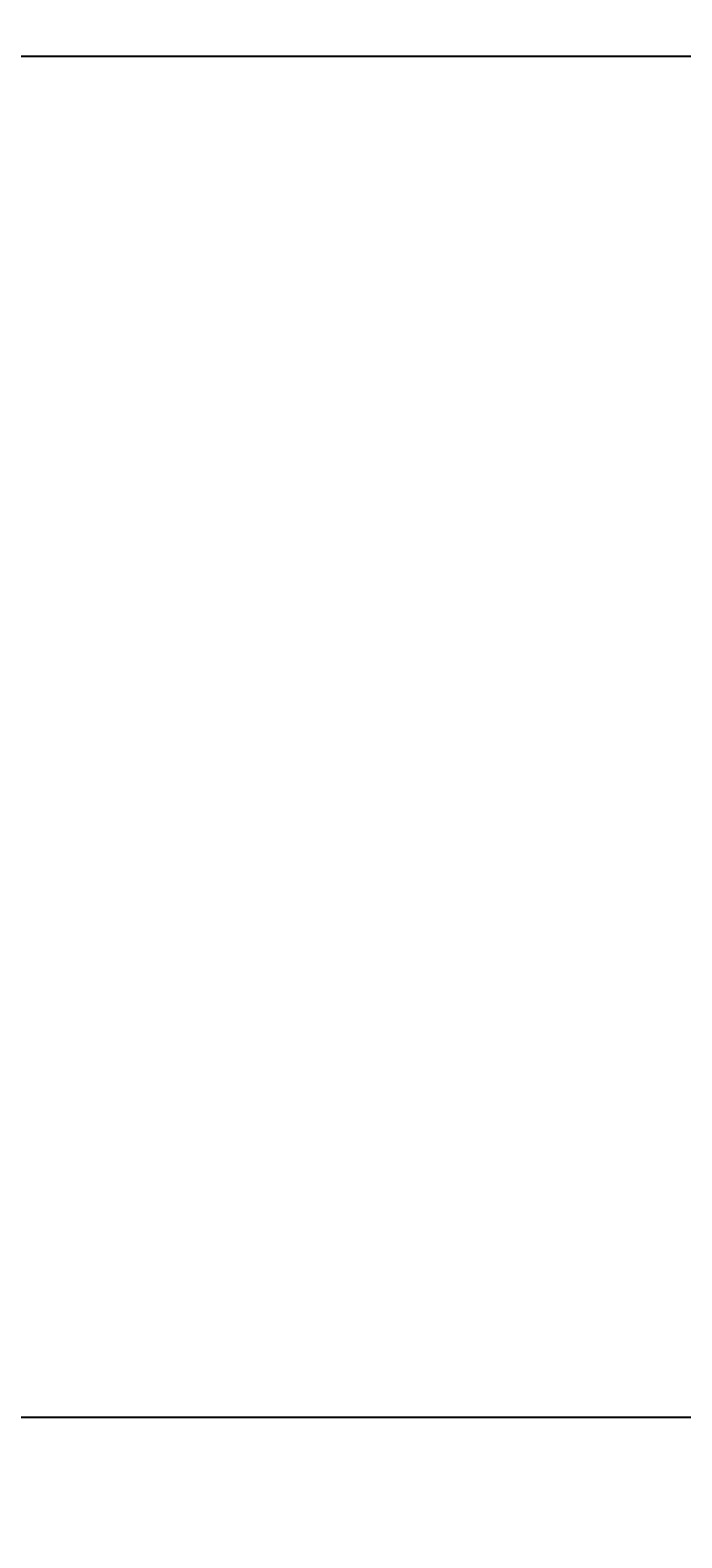
# Model space of a CAD drawing. Units: inches. Extents: x 35362 to 73946, y 43607 to 67532.
# Tile 52 of 134: x 49711 to 49915, y 46091 to 46564. Entities that reach past the tile are written whole.
import ezdxf

# ---------------------------------------------------------------- set-up
doc = ezdxf.new("R2010")
doc.units = ezdxf.units.IN
doc.header["$MEASUREMENT"] = 0
doc.layers.add('A-ANNO-DIMS', color=2, linetype='Continuous', lineweight=18)
doc.styles.get("Standard").update_dxf_attribs({"font": 'arial.ttf'})
doc.dimstyles.get("Standard").update_dxf_attribs({"dimtxt": 0.18, "dimasz": 0.18, "dimexe": 0.18, "dimexo": 0.0625, "dimgap": 0.09, "dimtad": 0, "dimtih": 1, "dimtoh": 1, "dimdec": 4, "dimzin": 0, "dimdsep": 46, "dimtxsty": 'Standard', "dimcen": 0.09, "dimadec": 0, "dimazin": 0, "dimtfac": 1, "dimtdec": 4, "dimtofl": 0, "dimtmove": 0, "dimatfit": 3, "dimfxl": 1, "dimtolj": 1, "dimtzin": 0, "dimarcsym": 0})

# ---------------------------------------------------------------- blocks, each defined once
blk = doc.blocks.new('*D5')
at = {"layer": 'A-ANNO-DIMS', "color": 0, "lineweight": -2, "transparency": 16777216}
for p, q in [((37121.95, 46919.32), (37121.95, 43606.68)), ((69871.5, 45449.83), (69871.5, 43606.68)), ((37122.13, 43606.86), (53496.29, 43606.86)), ((69871.32, 43606.86), (53497.15, 43606.86))]:
    blk.add_line(p, q, dxfattribs=at)
at = {"layer": 'A-ANNO-DIMS', "color": 0, "transparency": 16777216}
for points in [[(37122.13, 43606.89), (37122.13, 43606.83), (37121.95, 43606.86)], [(69871.32, 43606.89), (69871.32, 43606.83), (69871.5, 43606.86)]]:
    blk.add_solid(points, dxfattribs=at)
at = {"layer": 'Defpoints', "color": 0, "transparency": 16777216}
for p in [(37121.95, 46919.38), (69871.5, 45449.89), (69871.5, 43606.86)]:
    blk.add_point(p, dxfattribs=at)
at = {"layer": 'A-ANNO-DIMS', "color": 0, "transparency": 16777216, "insert": (53496.72, 43606.86), "char_height": 0.18, "attachment_point": 5}
blk.add_mtext('\\A1;32750', dxfattribs=at)
blk = doc.blocks.new('*D11')
at = {"layer": 'A-ANNO-DIMS', "color": 0, "lineweight": -2, "transparency": 16777216}
for p, q in [((47978.66, 56028.77), (47978.66, 43606.68)), ((53109.76, 56028.77), (53109.76, 43606.68)), ((47978.84, 43606.86), (50543.87, 43606.86)), ((53109.58, 43606.86), (50544.55, 43606.86))]:
    blk.add_line(p, q, dxfattribs=at)
at = {"layer": 'A-ANNO-DIMS', "color": 0, "transparency": 16777216}
for points in [[(47978.84, 43606.89), (47978.84, 43606.83), (47978.66, 43606.86)], [(53109.58, 43606.89), (53109.58, 43606.83), (53109.76, 43606.86)]]:
    blk.add_solid(points, dxfattribs=at)
at = {"layer": 'Defpoints', "color": 0, "transparency": 16777216}
for p in [(47978.66, 56028.84), (53109.76, 56028.84), (53109.76, 43606.86)]:
    blk.add_point(p, dxfattribs=at)
at = {"layer": 'A-ANNO-DIMS', "color": 0, "transparency": 16777216, "insert": (50544.21, 43606.86), "char_height": 0.18, "attachment_point": 5}
blk.add_mtext('\\A1;5131', dxfattribs=at)
blk = doc.blocks.new('*D13')
at = {"layer": 'A-ANNO-DIMS', "color": 0, "lineweight": -2, "transparency": 16777216}
for p, q in [((48373.49, 51694.02), (48373.49, 43606.68)), ((51029.04, 51694.02), (51029.04, 43606.68)), ((48373.67, 43606.86), (49700.8, 43606.86)), ((51028.86, 43606.86), (49701.73, 43606.86))]:
    blk.add_line(p, q, dxfattribs=at)
at = {"layer": 'A-ANNO-DIMS', "color": 0, "transparency": 16777216}
for points in [[(48373.67, 43606.89), (48373.67, 43606.83), (48373.49, 43606.86)], [(51028.86, 43606.89), (51028.86, 43606.83), (51029.04, 43606.86)]]:
    blk.add_solid(points, dxfattribs=at)
at = {"layer": 'Defpoints', "color": 0, "transparency": 16777216}
for p in [(48373.49, 51694.09), (51029.04, 51694.09), (51029.04, 43606.86)]:
    blk.add_point(p, dxfattribs=at)
at = {"layer": 'A-ANNO-DIMS', "color": 0, "transparency": 16777216, "insert": (49701.27, 43606.86), "char_height": 0.18, "attachment_point": 5}
blk.add_mtext('\\A1;2655.6', dxfattribs=at)
blk = doc.blocks.new('*D67')
at = {"layer": 'A-ANNO-DIMS', "color": 0, "lineweight": -2, "transparency": 16777216}
for p, q in [((56873.54, 53351.53), (35361.77, 53351.53)), ((35361.95, 53351.35), (35361.95, 49400.89)), ((35361.95, 45450.07), (35361.95, 49400.53)), ((53793.58, 45449.89), (35361.77, 45449.89))]:
    blk.add_line(p, q, dxfattribs=at)
at = {"layer": 'A-ANNO-DIMS', "color": 0, "transparency": 16777216}
for points in [[(35361.92, 53351.35), (35361.98, 53351.35), (35361.95, 53351.53)], [(35361.92, 45450.07), (35361.98, 45450.07), (35361.95, 45449.89)]]:
    blk.add_solid(points, dxfattribs=at)
at = {"layer": 'Defpoints', "color": 0, "transparency": 16777216}
for p in [(35361.95, 53351.53), (56873.6, 53351.53), (53793.64, 45449.89)]:
    blk.add_point(p, dxfattribs=at)
at = {"layer": 'A-ANNO-DIMS', "color": 0, "transparency": 16777216, "insert": (35361.95, 49400.71), "char_height": 0.18, "attachment_point": 5}
blk.add_mtext('\\A1;7901.6', dxfattribs=at)
blk = doc.blocks.new('*D76')
at = {"layer": 'A-ANNO-DIMS', "color": 0, "lineweight": -2, "transparency": 16777216}
for p, q in [((54052.84, 46555.29), (35361.77, 46555.29)), ((35361.95, 46555.11), (35361.95, 46342.27)), ((35361.95, 46129.06), (35361.95, 46341.9)), ((53793.58, 46128.88), (35361.77, 46128.88))]:
    blk.add_line(p, q, dxfattribs=at)
at = {"layer": 'A-ANNO-DIMS', "color": 0, "transparency": 16777216}
for points in [[(35361.92, 46555.11), (35361.98, 46555.11), (35361.95, 46555.29)], [(35361.92, 46129.06), (35361.98, 46129.06), (35361.95, 46128.88)]]:
    blk.add_solid(points, dxfattribs=at)
at = {"layer": 'Defpoints', "color": 0, "transparency": 16777216}
for p in [(35361.95, 46555.29), (54052.9, 46555.29), (53793.64, 46128.88)]:
    blk.add_point(p, dxfattribs=at)
at = {"layer": 'A-ANNO-DIMS', "color": 0, "transparency": 16777216, "insert": (35361.95, 46342.09), "char_height": 0.18, "attachment_point": 5}
blk.add_mtext('\\A1;426.4', dxfattribs=at)
blk = doc.blocks.new('*D90')
at = {"layer": 'A-ANNO-DIMS', "color": 0, "lineweight": -2, "transparency": 16777216}
for p, q in [((53707.72, 47291.29), (35361.77, 47291.29)), ((35361.95, 47291.11), (35361.95, 46710.26)), ((35361.95, 46129.06), (35361.95, 46709.9)), ((53793.58, 46128.88), (35361.77, 46128.88))]:
    blk.add_line(p, q, dxfattribs=at)
at = {"layer": 'A-ANNO-DIMS', "color": 0, "transparency": 16777216}
for points in [[(35361.92, 47291.11), (35361.98, 47291.11), (35361.95, 47291.29)], [(35361.92, 46129.06), (35361.98, 46129.06), (35361.95, 46128.88)]]:
    blk.add_solid(points, dxfattribs=at)
at = {"layer": 'Defpoints', "color": 0, "transparency": 16777216}
for p in [(53707.78, 47291.29), (35361.95, 46128.88), (53793.64, 46128.88)]:
    blk.add_point(p, dxfattribs=at)
at = {"layer": 'A-ANNO-DIMS', "color": 0, "transparency": 16777216, "insert": (35361.95, 46710.08), "char_height": 0.18, "attachment_point": 5}
blk.add_mtext('\\A1;1162.4', dxfattribs=at)

msp = doc.modelspace()

# ---------------------------------------------------------------- dimensions: what is measured, and where the dimension line sits
at = {"layer": 'A-ANNO-DIMS'}
for base, p1, p2, override, picture, middle in [((53109.76, 43606.859), (47978.665, 56028.836), (53109.76, 56028.836), {"dimdec": 0, "dimlfac": 1, "dimrnd": 0, "dimzin": 0, "dimdsep": 46, "dimlunit": 2}, '*D11', (50544.212, 43606.859)), ((51029.043, 43606.859), (48373.492, 51694.087), (51029.043, 51694.087), {"dimdec": 1, "dimlfac": 1, "dimrnd": 0, "dimzin": 0, "dimdsep": 46, "dimlunit": 2}, '*D13', (49701.267, 43606.859)), ((69871.496, 43606.859), (37121.949, 46919.381), (69871.496, 45449.894), {"dimdec": 0, "dimlfac": 1, "dimrnd": 0, "dimzin": 0, "dimdsep": 46, "dimlunit": 2}, '*D5', (53496.723, 43606.859))]:
    dim = msp.add_linear_dim(base=base, p1=p1, p2=p2, dimstyle='Standard', override=override, dxfattribs=at)
    dim.commit()
    dim.dimension.update_dxf_attribs({"geometry": picture, "text_midpoint": middle})
for base, p1, p2, picture, middle in [((35361.949, 53351.529), (53793.638, 45449.894), (56873.602, 53351.529), '*D67', (35361.949, 49400.712)), ((35361.949, 46128.878), (53707.781, 47291.285), (53793.638, 46128.878), '*D90', (35361.949, 46710.081)), ((35361.949, 46555.293), (53793.638, 46128.878), (54052.899, 46555.293), '*D76', (35361.949, 46342.086))]:
    dim = msp.add_linear_dim(base=base, p1=p1, p2=p2, angle=90, dimstyle='Standard', override={"dimdec": 1, "dimlfac": 1, "dimrnd": 0, "dimzin": 0, "dimdsep": 46, "dimlunit": 2}, dxfattribs=at)
    dim.commit()
    dim.dimension.update_dxf_attribs({"geometry": picture, "text_midpoint": middle})

doc.saveas('drawing.dxf')
